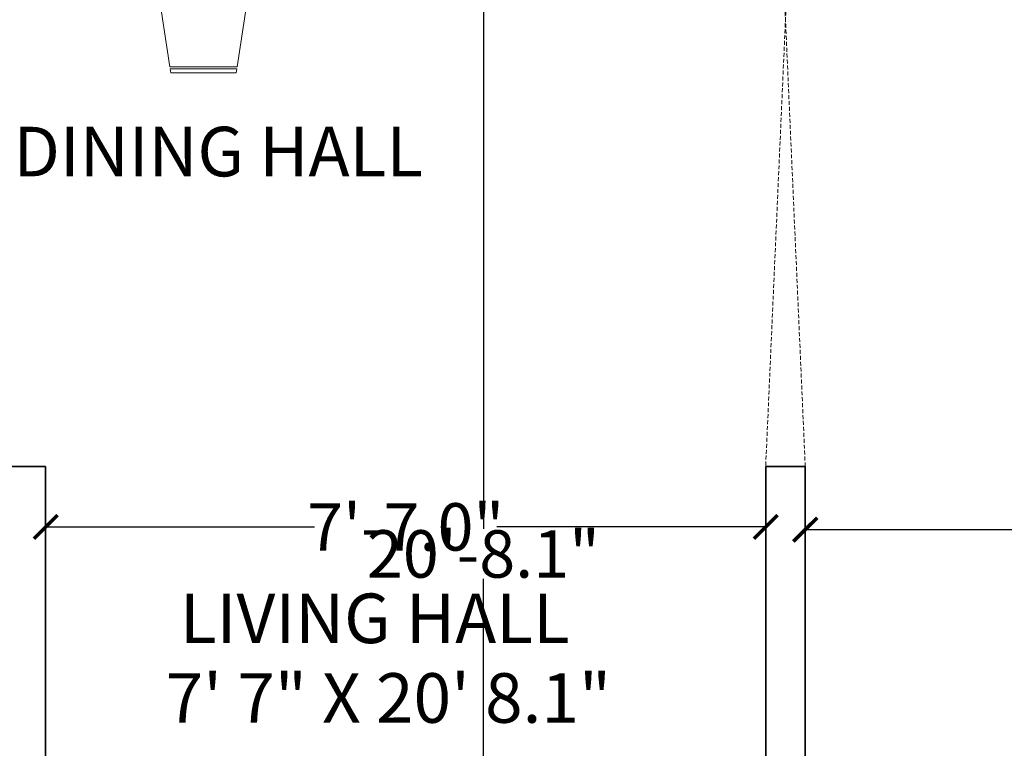
# Model space of a CAD drawing. Units: inches. Extents: x 844 to 2234, y 346 to 1084.
# Tile 65 of 93: x 1840 to 1964, y 736 to 828. Entities that reach past the tile are written whole.
import ezdxf

# ---------------------------------------------------------------- set-up
doc = ezdxf.new("R2010")
doc.units = ezdxf.units.IN
doc.header["$MEASUREMENT"] = 0
doc.linetypes.add('DASHED', pattern=[0.75, 0.5, -0.25])
for name, color, linetype, lineweight in [('A-ANNO-DIMS', 2, 'Continuous', 18), ('A-AREA-IDEN', 7, 'Continuous', 18), ('A-WALL', 7, 'Continuous', 35), ('A-WALL-OVHD', 7, 'DASHED', 18), ('furniture', 8, 'Continuous', 18)]:
    doc.layers.add(name, color=color, linetype=linetype, lineweight=lineweight)
doc.styles.add('ATTR', font='romans.shx', dxfattribs={"width": 0.8, "height": 0.7})
doc.styles.get("Standard").update_dxf_attribs({"font": 'arial.ttf'})
doc.dimstyles.get("Standard").update_dxf_attribs({"dimtxt": 6, "dimasz": 3, "dimexe": 0.18, "dimexo": 0.0625, "dimgap": 0.09, "dimtad": 0, "dimtih": 1, "dimtoh": 1, "dimdec": 1, "dimzin": 0, "dimdsep": 46, "dimlunit": 3, "dimtxsty": 'Standard', "dimblk": 'ARCHTICK', "dimcen": 0.09, "dimadec": 0, "dimazin": 0, "dimtfac": 1, "dimtdec": 1, "dimtofl": 0, "dimtmove": 0, "dimatfit": 3, "dimfxl": 1, "dimtolj": 1, "dimtzin": 0, "dimarcsym": 0})

# ---------------------------------------------------------------- blocks, each defined once
blk = doc.blocks.new('DIN42X84')
for p, q in [((-34.772, 36.500609), (-37.0377, 21.999999)), ((-34.7681, 36.499999), (-18.2986, 36.499999)), ((-34.5377, 37.999999), (-34.6939, 37.000439)), ((-18.3793, 36.999999), (-34.6911, 36.999999)), ((-34.5377, 37.999999), (-18.5377, 37.999999)), ((-18.3814, 36.999659), (-18.5377, 37.999999)), ((-16.0377, 21.999999), (-18.3032, 36.499269)), ((-8.2343, 36.500609), (-10.5001, 21.999999)), ((-8.2305, 36.499999), (8.2391, 36.499999)), ((-8.0001, 37.999999), (-8.1562, 37.000439)), ((8.1584, 36.999999), (-8.1535, 36.999999)), ((-8.0001, 37.999999), (7.9999, 37.999999)), ((8.1562, 36.999659), (7.9999, 37.999999)), ((10.4999, 21.999999), (8.2344, 36.499269)), ((16.0376, 21.999999), (18.3031, 36.499269)), ((34.768, 36.499999), (18.2985, 36.499999)), ((18.3792, 36.999999), (34.691, 36.999999)), ((18.3813, 36.999659), (18.5376, 37.999999)), ((34.5376, 37.999999), (18.5376, 37.999999)), ((34.5376, 37.999999), (34.6938, 37.000439)), ((34.7719, 36.500609), (37.0376, 21.999999)), ((-43, 10.499989), (-57.4993, 8.234489)), ((43, 10.499989), (57.4992, 8.234489)), ((-57.9997, 8.156299), (-59, 7.999989)), ((-59, -8.000011), (-59, 7.999989)), ((-58, 8.158429), (-58, -8.153391)), ((-57.5, -8.230411), (-57.5, 8.239139)), ((57.5, -8.230411), (57.5, 8.239139)), ((57.9996, 8.156299), (59, 7.999989)), ((58, 8.158429), (58, -8.153391)), ((59, -8.000011), (59, 7.999989)), ((-59, -8.000011), (-58.0005, -8.156181)), ((-57.5007, -8.234271), (-43, -10.500011)), ((57.5006, -8.234271), (43, -10.500011)), ((59, -8.000011), (58.0004, -8.156181)), ((-42, -21.000001), (42, -21.000001)), ((-34.772, -36.50061), (-37.0377, -22.000001)), ((-16.0377, -22.000001), (-18.3032, -36.499267)), ((-8.2343, -36.50061), (-10.5001, -22.000001)), ((10.4999, -22.000001), (8.2344, -36.499267)), ((16.0376, -22.000001), (18.3031, -36.499267)), ((34.7719, -36.50061), (37.0376, -22.000001)), ((-34.7681, -36.499999), (-18.2986, -36.499999)), ((-34.5377, -37.999999), (-34.6939, -37.000442)), ((-18.3793, -36.999999), (-34.6911, -36.999999)), ((-34.5377, -37.999999), (-18.5377, -37.999999)), ((-18.3814, -36.999664), (-18.5377, -37.999999)), ((-8.2305, -36.499999), (8.2391, -36.499999)), ((-8.0001, -37.999999), (-8.1562, -37.000442)), ((8.1584, -36.999999), (-8.1535, -36.999999)), ((-8.0001, -37.999999), (7.9999, -37.999999)), ((8.1562, -36.999664), (7.9999, -37.999999)), ((34.768, -36.499999), (18.2985, -36.499999)), ((18.3792, -36.999999), (34.691, -36.999999)), ((18.3813, -36.999664), (18.5376, -37.999999)), ((34.5376, -37.999999), (18.5376, -37.999999)), ((34.5376, -37.999999), (34.6938, -37.000442))]:
    blk.add_line(p, q)
for points in [[(-42, -21.000001), (-42, 20.999989), (42, 20.999989), (42, -21.000001)], [(-42, 16.999989), (-40.5974, 16.672209), (-39.2569, 16.395939), (-37.9668, 16.166109), (-36.7153, 15.977689), (-35.4906, 15.825599), (-34.281, 15.704799), (-33.0745, 15.610229), (-31.8595, 15.536839), (-30.6267, 15.480229), (-29.3778, 15.438619), (-28.117, 15.410889), (-26.8486, 15.395929), (-25.5767, 15.392599), (-24.3058, 15.399809), (-23.0399, 15.416409), (-21.7833, 15.441309), (-20.5384, 15.473619), (-19.2994, 15.513549), (-18.0587, 15.561549), (-16.8087, 15.618049), (-15.5417, 15.683499), (-14.25, 15.758369), (-12.9261, 15.843079), (-11.5622, 15.938089), (-10.1541, 16.043559), (-8.7108, 16.158419), (-7.2445, 16.281349), (-5.7675, 16.410999), (-4.2923, 16.546019), (-2.8311, 16.685069), (-1.3963, 16.826809), (0, 16.969889), (1.3474, 17.113339), (2.6447, 17.257689), (3.8928, 17.403829), (5.0924, 17.552659), (6.2444, 17.705069), (7.3498, 17.861959), (8.4092, 18.024219), (9.4237, 18.192759), (10.3952, 18.367629), (11.3311, 18.545639), (12.2397, 18.722759), (13.1297, 18.894949), (14.0095, 19.058179), (14.8876, 19.208429), (15.7725, 19.341659), (16.6727, 19.453839), (17.5977, 19.541909), (18.5617, 19.606689), (19.5795, 19.649979), (20.6664, 19.673569), (21.8374, 19.679239), (23.1076, 19.668789), (24.492, 19.644009), (26.0058, 19.606689), (27.6589, 19.554579), (29.4413, 19.469229), (31.3377, 19.328169), (33.3331, 19.108889), (35.4121, 18.788919), (37.5598, 18.345779), (39.7608, 17.756959), (42, 16.999989)], [(42, 12.999999), (39.3635, 13.704689), (36.9303, 14.232849), (34.6868, 14.608169), (32.6195, 14.854319), (30.7149, 14.994989), (28.9596, 15.053859), (27.34, 15.054629), (25.8427, 15.020959), (24.4543, 14.972439), (23.1628, 14.912279), (21.9562, 14.839589), (20.8227, 14.753449), (19.7504, 14.652989), (18.7273, 14.537299), (17.7416, 14.405489), (16.7814, 14.256669), (15.8348, 14.090369), (14.8899, 13.907959), (13.9348, 13.711209), (12.9575, 13.501929), (11.9464, 13.281899), (10.8893, 13.052909), (9.7745, 12.816759), (8.59, 12.575229), (7.3261, 12.330049), (5.9815, 12.082619), (4.557, 11.834299), (3.0536, 11.586429), (1.472, 11.340349), (-0.187, 11.097409), (-1.9223, 10.858939), (-3.7333, 10.626289), (-5.6141, 10.400739), (-7.539, 10.183249), (-9.4776, 9.974709), (-11.3991, 9.776019), (-13.2731, 9.588079), (-15.0689, 9.411789), (-16.756, 9.248039), (-18.3038, 9.097709), (-19.6928, 8.961719), (-20.9483, 8.840959), (-22.1065, 8.736319), (-23.2037, 8.648689), (-24.2763, 8.578979), (-25.3606, 8.528079), (-26.4928, 8.496879), (-27.7094, 8.486279), (-29.0411, 8.496689), (-30.4965, 8.526549), (-32.0787, 8.573829), (-33.7908, 8.636479), (-35.6359, 8.712459), (-37.6171, 8.799739), (-39.7374, 8.896259), (-42, 8.999999)], [(-42, 0.999999), (-39.2567, 1.059739), (-36.6668, 1.127399), (-34.2177, 1.203389), (-31.897, 1.288099), (-29.6923, 1.381949), (-27.5912, 1.485329), (-25.5812, 1.598659), (-23.65, 1.722319), (-21.7874, 1.856519), (-19.9935, 2.000569), (-18.2704, 2.153579), (-16.6207, 2.314649), (-15.0465, 2.482879), (-13.5503, 2.657379), (-12.1344, 2.837259), (-10.8011, 3.021619), (-9.5514, 3.209479), (-8.3812, 3.399579), (-7.2848, 3.590579), (-6.2569, 3.781129), (-5.2918, 3.969889), (-4.384, 4.155509), (-3.5281, 4.336659), (-2.7184, 4.511979), (-1.9505, 4.680359), (-1.2233, 4.841579), (-0.5369, 4.995629), (0.1087, 5.142519), (0.7135, 5.282239), (1.2776, 5.414799), (1.8009, 5.540189), (2.2834, 5.658409), (2.7259, 5.769699), (3.1323, 5.875159), (3.5073, 5.976139), (3.8555, 6.073989), (4.1816, 6.170049), (4.4904, 6.265659), (4.7863, 6.362169), (5.0742, 6.460919), (5.3584, 6.563099), (5.6417, 6.669299), (5.9267, 6.779989), (6.216, 6.895609), (6.512, 7.016589), (6.8174, 7.143399), (7.1347, 7.276479), (7.4664, 7.416279), (7.8159, 7.563169), (8.1896, 7.717219), (8.5948, 7.878439), (9.0386, 8.046819), (9.5282, 8.222369), (10.071, 8.405079), (10.674, 8.594959), (11.3446, 8.791999), (12.0866, 8.995459), (12.8902, 9.201609), (13.7421, 9.405969), (14.6294, 9.604059), (15.5387, 9.791399), (16.4569, 9.963509), (17.3709, 10.115919), (18.2674, 10.244149), (19.1361, 10.344989), (19.9772, 10.420299), (20.7936, 10.473209), (21.5884, 10.506879), (22.3645, 10.524419), (23.1248, 10.528969), (23.8725, 10.523669), (24.6103, 10.511649), (25.3403, 10.495379), (26.0601, 10.474629), (26.7663, 10.448509), (27.4556, 10.416119), (28.1244, 10.376559), (28.7695, 10.328939), (29.3873, 10.272359), (29.9746, 10.205939), (30.5293, 10.129059), (31.0552, 10.042329), (31.5572, 9.946639), (32.0406, 9.842899), (32.5104, 9.731989), (32.9716, 9.614799), (33.4295, 9.492249), (33.8891, 9.365219), (34.3546, 9.234229), (34.8266, 9.098309), (35.3051, 8.956129), (35.7897, 8.806329), (36.2802, 8.647569), (36.7765, 8.478519), (37.2783, 8.297819), (37.7854, 8.104139), (38.2976, 7.894309), (38.8146, 7.657969), (39.3361, 7.382899), (39.8617, 7.056919), (40.3912, 6.667829), (40.9243, 6.203449), (41.4607, 5.651569), (42, 4.999999)], [(42, 0.999999), (35.1214, 2.295539), (25.1178, 2.983399), (7.9376, 2.295539), (0.3261, 1.149099), (-6.6329, -0.226611), (-18.3763, -2.978061), (-22.0733, -3.895201), (-27.5101, -4.583071), (-32.9468, -4.583071), (-35.339, -4.583071), (-38.3836, -4.353771), (-40.3408, -3.665921), (-42, -3.000001)], [(42, -3.000001), (38.9344, -2.781351), (35.8829, -2.650251), (32.8567, -2.595491), (29.8672, -2.605821), (26.9257, -2.670031), (24.0436, -2.776881), (21.2323, -2.915141), (18.5031, -3.073591), (15.8668, -3.242611), (13.3327, -3.419021), (10.9095, -3.601241), (8.6059, -3.787731), (6.4305, -3.976901), (4.3921, -4.167191), (2.4994, -4.357031), (0.7611, -4.544851), (-0.8196, -4.729651), (-2.2614, -4.912671), (-3.5885, -5.095681), (-4.8252, -5.280481), (-5.9956, -5.468861), (-7.1239, -5.662621), (-8.2344, -5.863551), (-9.3513, -6.073431), (-10.4925, -6.293091), (-11.6511, -6.519461), (-12.814, -6.748531), (-13.968, -6.976251), (-15.0999, -7.198591), (-16.1965, -7.411531), (-17.2447, -7.611041), (-18.2313, -7.793081), (-19.1472, -7.954521), (-19.9994, -8.095811), (-20.7989, -8.218291), (-21.5568, -8.323311), (-22.2841, -8.412201), (-22.9919, -8.486311), (-23.6912, -8.546991), (-24.393, -8.595581), (-25.1087, -8.632751), (-25.8513, -8.656491), (-26.6337, -8.664101), (-27.4693, -8.652901), (-28.3711, -8.620211), (-29.3523, -8.563341), (-30.4262, -8.479601), (-31.6057, -8.366301), (-32.8956, -8.222561), (-34.2657, -8.054761), (-35.6772, -7.871051), (-37.0913, -7.679611), (-38.4695, -7.488621), (-39.7728, -7.306241), (-40.9626, -7.140641), (-42, -7.000001)], [(-42, -15.000001), (-38.4722, -15.350691), (-35.3039, -15.623741), (-32.4544, -15.828971), (-29.8831, -15.976191), (-27.5493, -16.075201), (-25.4123, -16.135831), (-23.4313, -16.167881), (-21.5659, -16.181151), (-19.7812, -16.183881), (-18.0665, -16.177871), (-16.4173, -16.163351), (-14.8288, -16.140551), (-13.2964, -16.109691), (-11.8154, -16.070991), (-10.3811, -16.024671), (-8.9888, -15.970971), (-7.6345, -15.909991), (-6.3163, -15.841401), (-5.0329, -15.764751), (-3.7831, -15.679591), (-2.5656, -15.585471), (-1.3791, -15.481951), (-0.2223, -15.368571), (0.9061, -15.244901), (2.0079, -15.110631), (3.0876, -14.966051), (4.1503, -14.811631), (5.2011, -14.647801), (6.2451, -14.475011), (7.2875, -14.293721), (8.3332, -14.104361), (9.3874, -13.907391), (10.4544, -13.703711), (11.5349, -13.495991), (12.6291, -13.287381), (13.7368, -13.081011), (14.8581, -12.880011), (15.9931, -12.687521), (17.1416, -12.506671), (18.3037, -12.340601), (19.4778, -12.191771), (20.6562, -12.059961), (21.8295, -11.944271), (22.9884, -11.843811), (24.1234, -11.757681), (25.2254, -11.684981), (26.2848, -11.624831), (27.2925, -11.576311), (28.2412, -11.538551), (29.1325, -11.510631), (29.9703, -11.491671), (30.7584, -11.480781), (31.5007, -11.477041), (32.2009, -11.479581), (32.8628, -11.487491), (33.4904, -11.499881), (34.0874, -11.515741), (34.6576, -11.533621), (35.2049, -11.551941), (35.733, -11.569151), (36.2459, -11.583661), (36.7473, -11.593931), (37.2411, -11.598371), (37.7311, -11.595421), (38.2211, -11.583281), (38.7152, -11.559251), (39.2177, -11.520361), (39.7326, -11.463671), (40.2641, -11.386241), (40.8164, -11.285111), (41.3937, -11.157351), (42, -11.000001)]]:
    blk.add_lwpolyline(points)
for centre, start, end in [((-36.0377, 21.999999), 180, 270), ((-17.0377, 21.999999), 270, 0), ((-9.5001, 21.999999), 180, 270), ((9.4999, 21.999999), 270, 0), ((17.0376, 21.999999), 180, 270), ((36.0376, 21.999999), 270, 0), ((-43, 9.499989), 0.00000068, 90), ((43, 9.499989), 90, 180), ((-43, -9.500011), 270, 0.00000068), ((43, -9.500011), 180, 270), ((-36.0377, -22.000001), 90, 180), ((-17.0377, -22.000001), 0, 90), ((-9.5001, -22.000001), 90, 180), ((9.4999, -22.000001), 0, 90), ((17.0376, -22.000001), 90, 180), ((36.0376, -22.000001), 0, 90)]:
    blk.add_arc(centre, 1, start, end)
at = {"style": 'ATTR', "width": 0.8, "flags": 9}
blk.add_attdef('ESTCODE', (0, 0), '', height=0.7, dxfattribs=at)
blk = doc.blocks.new('_ArchTick')
at = {"color": 0, "linetype": 'ByBlock', "const_width": 0.15}
blk.add_lwpolyline([(-0.5, -0.5), (0.5, 0.5)], dxfattribs=at)
blk = doc.blocks.new('*D80')
at = {"layer": 'A-ANNO-DIMS', "color": 0, "lineweight": -2, "transparency": 16777216}
for p, q in [((1939.1, 763.54), (1939.1, 763.65)), ((1939.1, 763.47), (1973.06, 763.47)), ((2030.1, 763.47), (1996.13, 763.47)), ((2030.1, 763.54), (2030.1, 763.65))]:
    blk.add_line(p, q, dxfattribs=at)
at = {"layer": 'Defpoints', "color": 0, "transparency": 16777216}
for p in [(1939.1, 763.47), (1939.1, 763.47), (2030.1, 763.47)]:
    blk.add_point(p, dxfattribs=at)
at = {"layer": 'A-ANNO-DIMS', "color": 0, "lineweight": -2, "transparency": 16777216, "xscale": 3, "yscale": 3, "zscale": 3, "rotation": 180}
blk.add_blockref('_ArchTick', (1939.1, 763.47), dxfattribs=at)
at = {"layer": 'A-ANNO-DIMS', "color": 0, "lineweight": -2, "transparency": 16777216, "xscale": 3, "yscale": 3, "zscale": 3}
blk.add_blockref('_ArchTick', (2030.1, 763.47), dxfattribs=at)
at = {"layer": 'A-ANNO-DIMS', "color": 0, "transparency": 16777216, "insert": (1984.6, 763.47), "char_height": 6, "attachment_point": 5}
blk.add_mtext('\\A1;7\'-7.0"', dxfattribs=at)
blk = doc.blocks.new('*D84')
at = {"layer": 'A-ANNO-DIMS', "color": 0, "lineweight": -2, "transparency": 16777216}
for p, q in [((1843.1, 763.81), (1877.06, 763.81)), ((1843.1, 763.75), (1843.1, 763.63)), ((1934.1, 763.81), (1900.13, 763.81)), ((1934.1, 763.87), (1934.1, 763.99))]:
    blk.add_line(p, q, dxfattribs=at)
at = {"layer": 'Defpoints', "color": 0, "transparency": 16777216}
for p in [(1843.1, 763.81), (1934.1, 763.81), (1934.1, 763.81)]:
    blk.add_point(p, dxfattribs=at)
at = {"layer": 'A-ANNO-DIMS', "color": 0, "lineweight": -2, "transparency": 16777216, "xscale": 3, "yscale": 3, "zscale": 3, "rotation": 180}
blk.add_blockref('_ArchTick', (1843.1, 763.81), dxfattribs=at)
at = {"layer": 'A-ANNO-DIMS', "color": 0, "lineweight": -2, "transparency": 16777216, "xscale": 3, "yscale": 3, "zscale": 3}
blk.add_blockref('_ArchTick', (1934.1, 763.81), dxfattribs=at)
at = {"layer": 'A-ANNO-DIMS', "color": 0, "transparency": 16777216, "insert": (1888.6, 763.81), "char_height": 6, "attachment_point": 5}
blk.add_mtext('\\A1;7\'-7.0"', dxfattribs=at)
blk = doc.blocks.new('*D85')
at = {"layer": 'A-ANNO-DIMS', "color": 0, "lineweight": -2, "transparency": 16777216}
for p, q in [((1886.16, 884.46), (1898.6, 884.46)), ((1898.42, 884.46), (1898.42, 763.55)), ((1898.42, 636.33), (1898.42, 757.24)), ((1886.16, 636.33), (1898.6, 636.33))]:
    blk.add_line(p, q, dxfattribs=at)
at = {"layer": 'Defpoints', "color": 0, "transparency": 16777216}
for p in [(1886.1, 884.46), (1886.1, 636.33), (1898.42, 636.33)]:
    blk.add_point(p, dxfattribs=at)
at = {"layer": 'A-ANNO-DIMS', "color": 0, "lineweight": -2, "transparency": 16777216, "xscale": 3, "yscale": 3, "zscale": 3}
for p, rotation in [((1898.42, 884.46), 90), ((1898.42, 636.33), 270)]:
    blk.add_blockref('_ArchTick', p, dxfattribs=dict(at, rotation=rotation))
at = {"layer": 'A-ANNO-DIMS', "color": 0, "transparency": 16777216, "insert": (1898.42, 760.39), "char_height": 6, "attachment_point": 5}
blk.add_mtext('\\A1;20\'-8.1"', dxfattribs=at)

msp = doc.modelspace()

# ---------------------------------------------------------------- linework, layer by layer
at = {"layer": 'A-WALL'}
for p, q in [((1838.1, 771.46), (1843.1, 771.46)), ((1843.1, 766.46), (1843.1, 771.46)), ((1934.1, 771.46), (1934.1, 634.46)), ((1934.1, 771.46), (1939.1, 771.46)), ((1939.1, 771.46), (1939.1, 634.46)), ((1843.1, 766.46), (1843.1, 629.46))]:
    msp.add_line(p, q, dxfattribs=at)
at = {"layer": 'A-WALL-OVHD'}
for p, q in [((1939.1, 771.46), (1934.1, 884.46)), ((1939.1, 884.46), (1934.1, 771.46))]:
    msp.add_line(p, q, dxfattribs=at)

# ---------------------------------------------------------------- block references
at = {"layer": 'furniture', "xscale": 0.5153672157522483, "yscale": 0.5153672157522483, "zscale": 0.5153672157522483, "rotation": 90}
msp.add_blockref('DIN42X84', (1863.05, 851.63), dxfattribs=at)

# ---------------------------------------------------------------- texts
at = {"layer": 'A-AREA-IDEN'}
for s, p in [('DINING HALL', (1839.02, 808.14)), ('LIVING HALL', (1860.06, 749.11)), (' 7\' 7" X 20\' 8.1"', (1856.36, 739.04))]:
    msp.add_text(s, height=6.2688, dxfattribs=at).set_placement(p)

# ---------------------------------------------------------------- dimensions: what is measured, and where the dimension line sits
at = {"layer": 'A-ANNO-DIMS'}
dim = msp.add_linear_dim(base=(1898.42, 636.33), p1=(1886.1, 884.46), p2=(1886.1, 636.33), angle=90, dimstyle='Standard', override={"dimclrd": 0, "dimclre": 0, "dimclrt": 0}, dxfattribs=at)
dim.commit()
dim.dimension.update_dxf_attribs({"geometry": '*D85', "text_midpoint": (1898.42, 760.39)})
for base, p1, p2, picture, middle in [((1934.1, 763.81), (1843.1, 763.81), (1934.1, 763.81), '*D84', (1888.6, 763.81)), ((1939.1, 763.47), (2030.1, 763.47), (1939.1, 763.47), '*D80', (1984.6, 763.47))]:
    dim = msp.add_linear_dim(base=base, p1=p1, p2=p2, dimstyle='Standard', override={"dimclrd": 0, "dimclre": 0, "dimclrt": 0}, dxfattribs=at)
    dim.commit()
    dim.dimension.update_dxf_attribs({"geometry": picture, "text_midpoint": middle})

doc.saveas('drawing.dxf')
